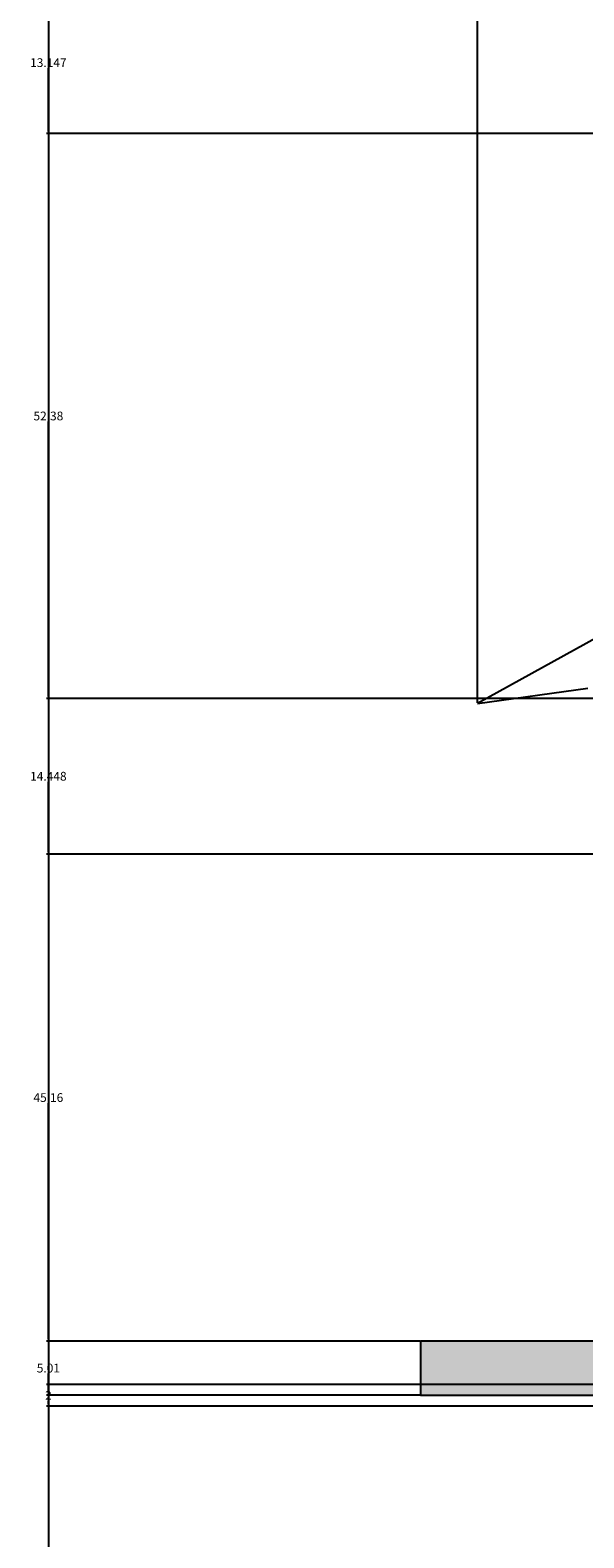
# Model space of a CAD drawing. Units: inches. Extents: x 36 to 594, y 79 to 831.
# Tile 20 of 30: x 36 to 87, y 590 to 730. Entities that reach past the tile are written whole.
import ezdxf

# ---------------------------------------------------------------- set-up
doc = ezdxf.new("R2010")
doc.units = ezdxf.units.IN
doc.header["$MEASUREMENT"] = 0
for name, color, linetype, lineweight in [('A-ANNO-DIMS', 2, 'Continuous', 18), ('A-ELEV', 7, 'Continuous', 25), ('A-ELEV-PATT', 8, 'Continuous', 13)]:
    doc.layers.add(name, color=color, linetype=linetype, lineweight=lineweight)
doc.styles.get("Standard").update_dxf_attribs({"font": 'arial.ttf'})
doc.dimstyles.get("Standard").update_dxf_attribs({"dimtxt": 0.8125, "dimasz": 0.18, "dimexe": 0.18, "dimexo": 0.0625, "dimgap": 0.09, "dimtad": 0, "dimtih": 1, "dimtoh": 1, "dimdec": 4, "dimzin": 0, "dimdsep": 46, "dimlunit": 4, "dimtxsty": 'Standard', "dimcen": 0.09, "dimadec": 0, "dimazin": 0, "dimtfac": 1, "dimtdec": 4, "dimtofl": 0, "dimtmove": 0, "dimatfit": 3, "dimfxl": 1, "dimtolj": 1, "dimtzin": 0, "dimarcsym": 0})

# ---------------------------------------------------------------- blocks, each defined once
blk = doc.blocks.new('*D12')
at = {"layer": 'A-ANNO-DIMS', "color": 0, "lineweight": -2, "transparency": 16777216}
for p, q in [((77.48, 667.8), (77.48, 830.73)), ((77.66, 830.55), (96.64, 830.55)), ((118.58, 830.55), (99.6, 830.55)), ((118.76, 594.27), (118.76, 830.73))]:
    blk.add_line(p, q, dxfattribs=at)
at = {"layer": 'A-ANNO-DIMS', "color": 0, "transparency": 16777216}
for points in [[(77.66, 830.58), (77.66, 830.52), (77.48, 830.55)], [(118.58, 830.58), (118.58, 830.52), (118.76, 830.55)]]:
    blk.add_solid(points, dxfattribs=at)
at = {"layer": 'Defpoints', "color": 0, "transparency": 16777216}
for p in [(118.76, 830.55), (77.48, 667.73), (118.76, 594.21)]:
    blk.add_point(p, dxfattribs=at)
at = {"layer": 'A-ANNO-DIMS', "color": 0, "transparency": 16777216, "insert": (98.12, 830.55), "char_height": 0.812, "attachment_point": 5}
blk.add_mtext('\\A1;41.28', dxfattribs=at)
blk = doc.blocks.new('*D21')
at = {"layer": 'A-ANNO-DIMS', "color": 0, "lineweight": -2, "transparency": 16777216}
for p, q in [((77.48, 667.8), (77.48, 830.73)), ((77.66, 830.55), (84.75, 830.55)), ((94.69, 830.55), (87.59, 830.55)), ((94.87, 668.27), (94.87, 830.73))]:
    blk.add_line(p, q, dxfattribs=at)
at = {"layer": 'A-ANNO-DIMS', "color": 0, "transparency": 16777216}
for points in [[(77.66, 830.58), (77.66, 830.52), (77.48, 830.55)], [(94.69, 830.58), (94.69, 830.52), (94.87, 830.55)]]:
    blk.add_solid(points, dxfattribs=at)
at = {"layer": 'Defpoints', "color": 0, "transparency": 16777216}
for p in [(94.87, 830.55), (77.48, 667.73), (94.87, 668.21)]:
    blk.add_point(p, dxfattribs=at)
at = {"layer": 'A-ANNO-DIMS', "color": 0, "transparency": 16777216, "insert": (86.17, 830.55), "char_height": 0.812, "attachment_point": 5}
blk.add_mtext('\\A1;17.39', dxfattribs=at)
blk = doc.blocks.new('*D28')
at = {"layer": 'A-ANNO-DIMS', "color": 0, "lineweight": -2, "transparency": 16777216}
for p, q in [((269.3, 796.05), (37.49, 796.05)), ((37.67, 795.87), (37.67, 455.63)), ((37.67, 114.39), (37.67, 454.62)), ((94.8, 114.21), (37.49, 114.21))]:
    blk.add_line(p, q, dxfattribs=at)
at = {"layer": 'A-ANNO-DIMS', "color": 0, "transparency": 16777216}
for points in [[(37.64, 795.87), (37.7, 795.87), (37.67, 796.05)], [(37.64, 114.39), (37.7, 114.39), (37.67, 114.21)]]:
    blk.add_solid(points, dxfattribs=at)
at = {"layer": 'Defpoints', "color": 0, "transparency": 16777216}
for p in [(37.67, 796.05), (269.36, 796.05), (94.87, 114.21)]:
    blk.add_point(p, dxfattribs=at)
at = {"layer": 'A-ANNO-DIMS', "color": 0, "transparency": 16777216, "insert": (37.67, 455.13), "char_height": 0.812, "attachment_point": 5}
blk.add_mtext('\\A1;681.8', dxfattribs=at)
blk = doc.blocks.new('*D44')
at = {"layer": 'A-ANNO-DIMS', "color": 0, "lineweight": -2, "transparency": 16777216}
for p, q in [((72.11, 603.6), (37.49, 603.6)), ((37.67, 603.42), (37.67, 513.6)), ((37.67, 422.77), (37.67, 512.59)), ((72.11, 422.59), (37.49, 422.59))]:
    blk.add_line(p, q, dxfattribs=at)
at = {"layer": 'A-ANNO-DIMS', "color": 0, "transparency": 16777216}
for points in [[(37.64, 603.42), (37.7, 603.42), (37.67, 603.6)], [(37.64, 422.77), (37.7, 422.77), (37.67, 422.59)]]:
    blk.add_solid(points, dxfattribs=at)
at = {"layer": 'Defpoints', "color": 0, "transparency": 16777216}
for p in [(37.67, 603.6), (72.17, 603.6), (72.17, 422.59)]:
    blk.add_point(p, dxfattribs=at)
at = {"layer": 'A-ANNO-DIMS', "color": 0, "transparency": 16777216, "insert": (37.67, 513.09), "char_height": 0.812, "attachment_point": 5}
blk.add_mtext('\\A1;181', dxfattribs=at)
blk = doc.blocks.new('*D45')
at = {"layer": 'A-ANNO-DIMS', "color": 0, "lineweight": -2, "transparency": 16777216}
for p, q in [((72.11, 608.61), (37.49, 608.61)), ((37.67, 608.43), (37.67, 606.61)), ((37.67, 603.78), (37.67, 605.6)), ((72.11, 603.6), (37.49, 603.6))]:
    blk.add_line(p, q, dxfattribs=at)
at = {"layer": 'A-ANNO-DIMS', "color": 0, "transparency": 16777216}
for points in [[(37.64, 608.43), (37.7, 608.43), (37.67, 608.61)], [(37.64, 603.78), (37.7, 603.78), (37.67, 603.6)]]:
    blk.add_solid(points, dxfattribs=at)
at = {"layer": 'Defpoints', "color": 0, "transparency": 16777216}
for p in [(37.67, 608.61), (72.17, 608.61), (72.17, 603.6)]:
    blk.add_point(p, dxfattribs=at)
at = {"layer": 'A-ANNO-DIMS', "color": 0, "transparency": 16777216, "insert": (37.67, 606.1), "char_height": 0.812, "attachment_point": 5}
blk.add_mtext('\\A1;5.01', dxfattribs=at)
blk = doc.blocks.new('*D46')
at = {"layer": 'A-ANNO-DIMS', "color": 0, "lineweight": -2, "transparency": 16777216}
for p, q in [((164.7, 653.76), (37.49, 653.76)), ((37.67, 653.58), (37.67, 631.69)), ((37.67, 608.79), (37.67, 630.68)), ((72.11, 608.61), (37.49, 608.61))]:
    blk.add_line(p, q, dxfattribs=at)
at = {"layer": 'A-ANNO-DIMS', "color": 0, "transparency": 16777216}
for points in [[(37.64, 653.58), (37.7, 653.58), (37.67, 653.76)], [(37.64, 608.79), (37.7, 608.79), (37.67, 608.61)]]:
    blk.add_solid(points, dxfattribs=at)
at = {"layer": 'Defpoints', "color": 0, "transparency": 16777216}
for p in [(37.67, 653.76), (164.77, 653.76), (72.17, 608.61)]:
    blk.add_point(p, dxfattribs=at)
at = {"layer": 'A-ANNO-DIMS', "color": 0, "transparency": 16777216, "insert": (37.67, 631.19), "char_height": 0.812, "attachment_point": 5}
blk.add_mtext('\\A1;45.16', dxfattribs=at)
blk = doc.blocks.new('*D47')
at = {"layer": 'A-ANNO-DIMS', "color": 0, "lineweight": -2, "transparency": 16777216}
for p, q in [((94.8, 668.21), (37.49, 668.21)), ((37.67, 668.03), (37.67, 661.49)), ((37.67, 653.94), (37.67, 660.48)), ((164.7, 653.76), (37.49, 653.76))]:
    blk.add_line(p, q, dxfattribs=at)
at = {"layer": 'A-ANNO-DIMS', "color": 0, "transparency": 16777216}
for points in [[(37.64, 668.03), (37.7, 668.03), (37.67, 668.21)], [(37.64, 653.94), (37.7, 653.94), (37.67, 653.76)]]:
    blk.add_solid(points, dxfattribs=at)
at = {"layer": 'Defpoints', "color": 0, "transparency": 16777216}
for p in [(37.67, 668.21), (94.87, 668.21), (164.77, 653.76)]:
    blk.add_point(p, dxfattribs=at)
at = {"layer": 'A-ANNO-DIMS', "color": 0, "transparency": 16777216, "insert": (37.67, 660.99), "char_height": 0.812, "attachment_point": 5}
blk.add_mtext('\\A1;14.448', dxfattribs=at)
blk = doc.blocks.new('*D48')
at = {"layer": 'A-ANNO-DIMS', "color": 0, "lineweight": -2, "transparency": 16777216}
for p, q in [((201.36, 720.59), (37.49, 720.59)), ((37.67, 720.41), (37.67, 694.91)), ((37.67, 668.39), (37.67, 693.9)), ((94.8, 668.21), (37.49, 668.21))]:
    blk.add_line(p, q, dxfattribs=at)
at = {"layer": 'A-ANNO-DIMS', "color": 0, "transparency": 16777216}
for points in [[(37.64, 720.41), (37.7, 720.41), (37.67, 720.59)], [(37.64, 668.39), (37.7, 668.39), (37.67, 668.21)]]:
    blk.add_solid(points, dxfattribs=at)
at = {"layer": 'Defpoints', "color": 0, "transparency": 16777216}
for p in [(37.67, 720.59), (201.42, 720.59), (94.87, 668.21)]:
    blk.add_point(p, dxfattribs=at)
at = {"layer": 'A-ANNO-DIMS', "color": 0, "transparency": 16777216, "insert": (37.67, 694.4), "char_height": 0.812, "attachment_point": 5}
blk.add_mtext('\\A1;52.38', dxfattribs=at)
blk = doc.blocks.new('*D49')
at = {"layer": 'A-ANNO-DIMS', "color": 0, "lineweight": -2, "transparency": 16777216}
for p, q in [((209.97, 733.74), (37.49, 733.74)), ((37.67, 733.56), (37.67, 727.67)), ((37.67, 720.77), (37.67, 726.66)), ((201.36, 720.59), (37.49, 720.59))]:
    blk.add_line(p, q, dxfattribs=at)
at = {"layer": 'A-ANNO-DIMS', "color": 0, "transparency": 16777216}
for points in [[(37.64, 733.56), (37.7, 733.56), (37.67, 733.74)], [(37.64, 720.77), (37.7, 720.77), (37.67, 720.59)]]:
    blk.add_solid(points, dxfattribs=at)
at = {"layer": 'Defpoints', "color": 0, "transparency": 16777216}
for p in [(37.67, 733.74), (210.03, 733.74), (201.42, 720.59)]:
    blk.add_point(p, dxfattribs=at)
at = {"layer": 'A-ANNO-DIMS', "color": 0, "transparency": 16777216, "insert": (37.67, 727.17), "char_height": 0.812, "attachment_point": 5}
blk.add_mtext('\\A1;13.147', dxfattribs=at)
blk = doc.blocks.new('*D122')
at = {"layer": 'A-ANNO-DIMS', "color": 0, "lineweight": -2, "transparency": 16777216}
for p, q in [((201.36, 604.57), (37.49, 604.57)), ((37.67, 604.39), (37.67, 604.06)), ((37.67, 602.75), (37.67, 603.07)), ((201.36, 602.57), (37.49, 602.57))]:
    blk.add_line(p, q, dxfattribs=at)
at = {"layer": 'A-ANNO-DIMS', "color": 0, "transparency": 16777216}
for points in [[(37.64, 604.39), (37.7, 604.39), (37.67, 604.57)], [(37.64, 602.75), (37.7, 602.75), (37.67, 602.57)]]:
    blk.add_solid(points, dxfattribs=at)
at = {"layer": 'Defpoints', "color": 0, "transparency": 16777216}
for p in [(37.67, 604.57), (201.42, 604.57), (201.42, 602.57)]:
    blk.add_point(p, dxfattribs=at)
at = {"layer": 'A-ANNO-DIMS', "color": 0, "transparency": 16777216, "insert": (37.67, 603.57), "char_height": 0.812, "attachment_point": 5}
blk.add_mtext('\\A1;2', dxfattribs=at)

msp = doc.modelspace()

# ---------------------------------------------------------------- hatches: boundary and pattern name
at = {"layer": 'A-ELEV-PATT'}
h = msp.add_hatch(color=256, dxfattribs=at)
h.dxf.hatch_style = 1
h.paths.add_polyline_path([(94.8658, 608.6081), (72.1733, 608.6081), (72.1733, 603.598), (94.8658, 603.598)])
h.paths.add_polyline_path([(94.8658, 427.5982), (72.1733, 427.5982), (72.1733, 422.5882), (94.8658, 422.5882)])
h.paths.add_polyline_path([(94.8658, 299.486), (72.1733, 299.486), (72.1733, 294.4759), (94.8658, 294.4759)])
h.paths.add_polyline_path([(269.3592, 770.1455), (260.5727, 770.1455), (260.5727, 764.0341), (269.3592, 764.0341)])
h.paths.add_polyline_path([(410.2381, 770.1455), (269.3592, 770.1455), (269.3592, 764.0341), (410.2381, 764.0341)])

# ---------------------------------------------------------------- linework, layer by layer
at = {"layer": 'A-ELEV'}
for p, q in [((91.3364, 675.3917), (77.477, 667.7335)), ((77.477, 667.7335), (87.7109, 669.1522))]:
    msp.add_line(p, q, dxfattribs=at)
msp.add_lwpolyline([(94.8658, 608.6081), (72.1733, 608.6081), (72.1733, 603.598), (94.8658, 603.598)], close=True, dxfattribs=at)

# ---------------------------------------------------------------- dimensions: what is measured, and where the dimension line sits
at = {"layer": 'A-ANNO-DIMS'}
for base, p2, picture, middle in [((118.7598, 830.5465), (118.7598, 594.2124), '*D12', (98.1184, 830.5465)), ((94.8658, 830.5465), (94.8658, 668.2124), '*D21', (86.1714, 830.5465))]:
    dim = msp.add_linear_dim(base=base, p1=(77.477, 667.7335), p2=p2, dimstyle='Standard', override={"dimdec": 2, "dimlfac": 1, "dimrnd": 0, "dimzin": 0, "dimdsep": 46, "dimlunit": 2}, dxfattribs=at)
    dim.commit()
    dim.dimension.update_dxf_attribs({"geometry": picture, "text_midpoint": middle})
for base, p1, p2, override, picture, middle in [((37.6733, 796.0465), (94.8658, 114.2124), (269.3592, 796.0465), {"dimdec": 1, "dimlfac": 1, "dimrnd": 0, "dimzin": 0, "dimdsep": 46, "dimlunit": 2}, '*D28', (37.6733, 455.1294)), ((37.6733, 733.7417), (201.4189, 720.595), (210.028, 733.7417), {"dimdec": 3, "dimlfac": 1, "dimrnd": 0, "dimzin": 0, "dimdsep": 46, "dimlunit": 2}, '*D49', (37.6733, 727.1683)), ((37.6733, 720.595), (94.8658, 668.2124), (201.4189, 720.595), {"dimdec": 2, "dimlfac": 1, "dimrnd": 0, "dimzin": 0, "dimdsep": 46, "dimlunit": 2}, '*D48', (37.6733, 694.4037)), ((37.6733, 668.2124), (164.7665, 653.7648), (94.8658, 668.2124), {"dimdec": 3, "dimlfac": 1, "dimrnd": 0, "dimzin": 0, "dimdsep": 46, "dimlunit": 2}, '*D47', (37.6733, 660.9886)), ((37.6733, 653.7648), (72.1733, 608.6081), (164.7665, 653.7648), {"dimdec": 2, "dimlfac": 1, "dimrnd": 0, "dimzin": 0, "dimdsep": 46, "dimlunit": 2}, '*D46', (37.6733, 631.1865)), ((37.6733, 608.6081), (72.1733, 603.598), (72.1733, 608.6081), {"dimdec": 2, "dimlfac": 1, "dimrnd": 0, "dimzin": 0, "dimdsep": 46, "dimlunit": 2}, '*D45', (37.6733, 606.1031)), ((37.6733, 604.5667), (201.4189, 602.5667), (201.4189, 604.5667), {"dimdec": 0, "dimlfac": 1, "dimrnd": 0, "dimzin": 0, "dimdsep": 46, "dimlunit": 2}, '*D122', (37.6733, 603.5667)), ((37.6733, 603.598), (72.1733, 422.5882), (72.1733, 603.598), {"dimdec": 0, "dimlfac": 1, "dimrnd": 0, "dimzin": 0, "dimdsep": 46, "dimlunit": 2}, '*D44', (37.6733, 513.0931))]:
    dim = msp.add_linear_dim(base=base, p1=p1, p2=p2, angle=90, dimstyle='Standard', override=override, dxfattribs=at)
    dim.commit()
    dim.dimension.update_dxf_attribs({"geometry": picture, "text_midpoint": middle})

doc.saveas('drawing.dxf')
